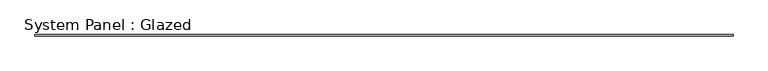
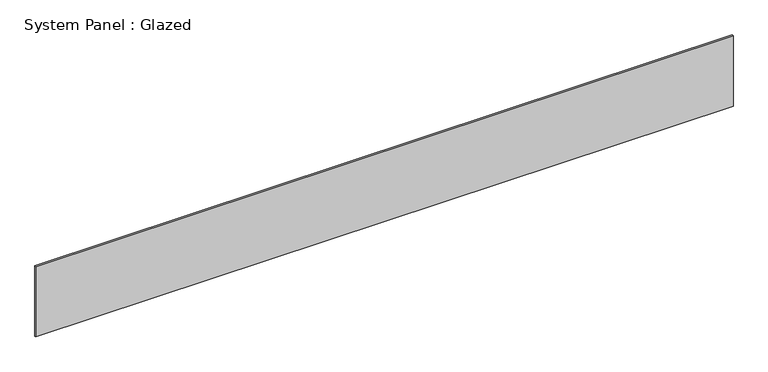
"""IFC4 building model written with IfcOpenShell, lengths in millimetres: plate geometry, System Panel : Glazed."""

from ifc_helpers import new_model, si_unit, origin, origin_with_axes, place, context, project, spatial, polyline, outline, extrude, source, transform, mapped, element, save


def system_panel_glazed_929cc49f(model_context):
    return source(origin(), model_context, "Body", "SweptSolid", [
        extrude(outline(polyline([(6845.7235748, 19.05), (-6845.7235748, 19.05), (-6845.7235748, 44.45), (6845.7235748, 44.45), (6845.7235748, 19.05)])), origin_with_axes(), (0.0, 0.0, 1.0), 1460.5),
    ])


if __name__ == "__main__":
    model = new_model("IFC4")
    model_context = context("Model", 3, world=origin())
    ifc_project = project(units=[si_unit("LENGTHUNIT", "METRE", prefix="MILLI")], contexts=[model_context])
    site = spatial("IfcSite", under=ifc_project)
    building = spatial("IfcBuilding", under=site)
    placement = place(None, origin())
    system_panel_glazed_shape = system_panel_glazed_929cc49f(model_context)
    element("IfcPlate", 1, ObjectType="System Panel : Glazed", at=placement, inside=building, context=model_context, shape_type="MappedRepresentation", body=[
        mapped(system_panel_glazed_shape, transform((0.0, 0.0, 0.0), x_axis=(1.0, 0.0, 0.0), y_axis=(0.0, 1.0, 0.0), z_axis=(0.0, 0.0, 1.0))),
    ])
    save(model, "model.ifc")

# Revit data of these elements
# Type "System Panel : Glazed"
#   Construction Type Id = "GSP4R"
#   Analytic Construction = "1/8 in Pilkington single glazing"
#   Visual Light Transmittance = 0.9
#   Solar Heat Gain Coefficient = 0.86
#   Heat Transfer Coefficient (U) = 1.18115 BTU/(h·ft²·°F)
# Element 1 (IfcPlate, "System Panel : Glazed")
#   Materials on its faces: "Glass"
# Materials
#   "Glass": class "Glass", colour RGB 0 128 192, transparency 0.75, Description = "Soda Lime Glass", Cost = 0
